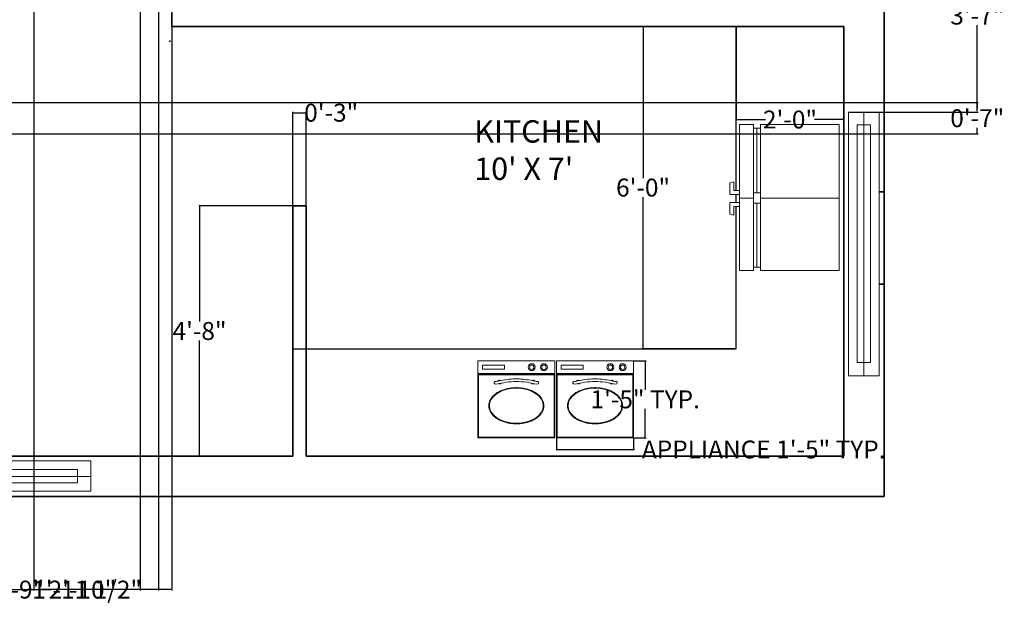
# Model space of a CAD drawing. Units: inches. Extents: x 311 to 754, y 60 to 497.
# Tile 6 of 11: x 530 to 750, y 60 to 194. Entities that reach past the tile are written whole.
import ezdxf

# ---------------------------------------------------------------- set-up
doc = ezdxf.new("R2010")
doc.units = ezdxf.units.IN
doc.header["$MEASUREMENT"] = 0
for name, color, linetype, lineweight in [('A-ANNO-DIMS', 2, 'Continuous', 18), ('A-AREA-IDEN', 1, 'Continuous', 18), ('A-EQPM', 8, 'Continuous', 18), ('A-FLOR-CASE', 30, 'Continuous', 25), ('A-WALL', 7, 'Continuous', 35), ('windows', 120, 'Continuous', 18)]:
    doc.layers.add(name, color=color, linetype=linetype, lineweight=lineweight)
doc.styles.get("Standard").update_dxf_attribs({"font": 'arial.ttf'})
doc.dimstyles.get("Standard").update_dxf_attribs({"dimtxt": 4, "dimasz": 0.18, "dimexe": 0.18, "dimexo": 0.0625, "dimgap": 0.09, "dimtad": 0, "dimtih": 1, "dimtoh": 1, "dimdec": 0, "dimrnd": 6, "dimzin": 0, "dimdsep": 46, "dimlunit": 3, "dimtxsty": 'Standard', "dimcen": 0.09, "dimadec": 0, "dimazin": 0, "dimtfac": 1, "dimtdec": 0, "dimtofl": 0, "dimtmove": 0, "dimatfit": 3, "dimfxl": 1, "dimtolj": 1, "dimtzin": 0, "dimarcsym": 0})

# ---------------------------------------------------------------- blocks, each defined once
blk = doc.blocks.new('A$C7E884C79')
for p, q in [((0, 0), (0, 600)), ((0, 600), (0, 0)), ((0, 600), (600, 600)), ((600, 600), (600, 0)), ((600, 0), (600, 600)), ((600, 600), (600, 450)), ((600, 600), (600, 500)), ((600, 500), (0, 500)), ((600, 495), (0, 495)), ((600, 500), (600, 0)), ((0, 0), (600, 0))]:
    blk.add_line(p, q)
for points in [[(36.4, 564.7), (208.9, 564.7), (208.9, 535.3), (36.4, 535.3)], [(5, 490), (595, 490), (595, 5), (5, 5)]]:
    blk.add_lwpolyline(points, close=True)
for centre, radius in [((419.3, 550), 27), ((419.3, 550), 17), ((513.9, 550), 27), ((513.9, 550), 17)]:
    blk.add_circle(centre, radius)
for centre, radius, start, end in [((137.2, 428), 10, 107.98291, 276.95811), ((168.5, 434.2), 15, 50.78881, 150.36701), ((168.5, 434.2), 15, 234.01645, 327.14121), ((431.5, 434.2), 15, 212.85879, 305.98355), ((431.5, 434.2), 15, 29.63299, 129.21119), ((462.8, 428), 10, 263.04189, 72.01709)]:
    blk.add_arc(centre, radius, start, end)
blk.add_ellipse((300, 250), major_axis=(-209.5, 0), ratio=0.648352)
for points, knots in [([(85.5, 250), (85.5, 244.8), (85.9, 239.6), (88, 226.9), (90.2, 219.4), (96.4, 204.8), (100.4, 197.7), (109.9, 184.1), (115.6, 177.5), (128.3, 165.1), (135.4, 159.2), (150.9, 148.3), (159.3, 143.3), (177.1, 134.2), (186.6, 130.1), (206.5, 123), (216.8, 119.9), (238.1, 114.9), (249, 113), (271.2, 110.2), (282.5, 109.4), (305, 109), (316.4, 109.4), (338.8, 111.3), (349.8, 112.8), (371.5, 117), (382.1, 119.6), (402.5, 126), (412.3, 129.7), (431, 138.1), (439.8, 142.8), (456.2, 153), (463.8, 158.6), (477.6, 170.5), (483.8, 176.8), (494.6, 190.1), (499.2, 197), (506.7, 211.3), (509.5, 218.7), (513.4, 233.6), (514.4, 241.3), (514.6, 256.5), (513.8, 264.1), (510.2, 279.1), (507.6, 286.6), (500.4, 300.9), (496, 307.9), (485.5, 321.3), (479.5, 327.7), (466, 339.7), (458.5, 345.3), (442.4, 355.8), (433.6, 360.5), (415.2, 369.1), (405.5, 373), (385.2, 379.5), (374.7, 382.3), (353.1, 386.7), (342, 388.3), (319.7, 390.5), (308.4, 390.9), (285.8, 390.7), (274.5, 390.1), (252.3, 387.5), (241.3, 385.7), (219.9, 380.9), (209.5, 378), (189.5, 371), (179.9, 367.1), (161.8, 358.1), (153.3, 353.2), (137.6, 342.5), (130.3, 336.7), (117.3, 324.4), (111.6, 317.9), (101.6, 304.3), (97.5, 297.3), (91, 282.8), (88.6, 275.3), (86, 261.9), (85.5, 255.9), (85.5, 250)], [0, 0, 0, 0, 0.108301, 0.108301, 0.267534, 0.267534, 0.426768, 0.426768, 0.586002, 0.586002, 0.745235, 0.745235, 0.904469, 0.904469, 1.063703, 1.063703, 1.222936, 1.222936, 1.38217, 1.38217, 1.541404, 1.541404, 1.700637, 1.700637, 1.859871, 1.859871, 2.019105, 2.019105, 2.178339, 2.178339, 2.337572, 2.337572, 2.496806, 2.496806, 2.65604, 2.65604, 2.815273, 2.815273, 2.974507, 2.974507, 3.133741, 3.133741, 3.292974, 3.292974, 3.452208, 3.452208, 3.611442, 3.611442, 3.770676, 3.770676, 3.929909, 3.929909, 4.089143, 4.089143, 4.248377, 4.248377, 4.40761, 4.40761, 4.566844, 4.566844, 4.726078, 4.726078, 4.885311, 4.885311, 5.044545, 5.044545, 5.203779, 5.203779, 5.363012, 5.363012, 5.522246, 5.522246, 5.68148, 5.68148, 5.840714, 5.840714, 5.999947, 5.999947, 6.159181, 6.159181, 6.283185, 6.283185, 6.283185, 6.283185]), ([(134.1, 437.5), (144.6, 439.5), (155.1, 441.6), (186, 447.3), (206.5, 450.9), (247.9, 456.4), (268.7, 458.3), (293.5, 458.9), (297.3, 458.9), (304.8, 458.9), (308.5, 458.8), (319.7, 458.5), (327.1, 458.1), (349.4, 456.5), (364.1, 454.9), (399.8, 449.9), (420.6, 446.2), (449.5, 440.7), (457.7, 439.1), (465.9, 437.5)], [0, 0, 0, 0, 31.638865, 31.638865, 92.600143, 92.600143, 153.561421, 153.561421, 164.367647, 164.367647, 175.173874, 175.173874, 196.786327, 196.786327, 240.011233, 240.011233, 302.099201, 302.099201, 326.773065, 326.773065, 326.773065, 326.773065])]:
    blk.add_open_spline(points, degree=3, knots=knots)
blk.add_open_spline([(138, 417.8), (192, 428.4), (300, 449.4), (408, 428.4), (462, 417.8)], degree=3)
blk = doc.blocks.new('WIN-FRAME-59IN')
for points in [[(0, 0), (0, 6.8), (58.92, 6.8), (58.92, 0)], [(2.85, 4.84), (55.97, 4.84), (55.97, 1.89), (2.85, 1.89)]]:
    blk.add_lwpolyline(points, close=True)
blk = doc.blocks.new('*D112')
at = {"layer": 'A-ANNO-DIMS', "color": 0, "lineweight": -2, "transparency": 16777216}
for p, q in [((649.67, 100.26), (649.67, 97.56)), ((666.89, 100.26), (666.89, 97.56)), ((649.85, 97.74), (666.71, 97.74)), ((666.89, 97.74), (667.07, 97.74))]:
    blk.add_line(p, q, dxfattribs=at)
at = {"layer": 'A-ANNO-DIMS', "color": 0, "transparency": 16777216}
for points in [[(649.85, 97.77), (649.85, 97.71), (649.67, 97.74)], [(666.71, 97.77), (666.71, 97.71), (666.89, 97.74)]]:
    blk.add_solid(points, dxfattribs=at)
at = {"layer": 'Defpoints', "color": 0, "transparency": 16777216}
for p in [(649.67, 100.33), (666.89, 100.33), (666.89, 97.74)]:
    blk.add_point(p, dxfattribs=at)
at = {"layer": 'A-ANNO-DIMS', "color": 0, "transparency": 16777216, "insert": (695.93, 97.74), "char_height": 4, "attachment_point": 5}
blk.add_mtext('\\A1;APPLIANCE 1\'-5" TYP.', dxfattribs=at)
blk = doc.blocks.new('*D113')
at = {"layer": 'A-ANNO-DIMS', "color": 0, "lineweight": -2, "transparency": 16777216}
for p, q in [((666.95, 117.55), (669.66, 117.55)), ((669.48, 117.37), (669.48, 111.07)), ((669.48, 100.51), (669.48, 106.81)), ((666.95, 100.33), (669.66, 100.33))]:
    blk.add_line(p, q, dxfattribs=at)
at = {"layer": 'A-ANNO-DIMS', "color": 0, "transparency": 16777216}
for points in [[(669.45, 117.37), (669.51, 117.37), (669.48, 117.55)], [(669.45, 100.51), (669.51, 100.51), (669.48, 100.33)]]:
    blk.add_solid(points, dxfattribs=at)
at = {"layer": 'Defpoints', "color": 0, "transparency": 16777216}
for p in [(666.89, 117.55), (669.48, 117.55), (666.89, 100.33)]:
    blk.add_point(p, dxfattribs=at)
at = {"layer": 'A-ANNO-DIMS', "color": 0, "transparency": 16777216, "insert": (669.48, 108.94), "char_height": 4, "attachment_point": 5}
blk.add_mtext('\\A1;1\'-5" TYP.', dxfattribs=at)
blk = doc.blocks.new('*D123')
at = {"layer": 'A-ANNO-DIMS', "color": 0, "lineweight": -2, "transparency": 16777216}
for p, q in [((715.13, 216.2), (743.78, 216.2)), ((743.6, 216.02), (743.6, 196.79)), ((743.6, 173.28), (743.6, 192.52)), ((714.96, 173.1), (743.78, 173.1))]:
    blk.add_line(p, q, dxfattribs=at)
at = {"layer": 'A-ANNO-DIMS', "color": 0, "transparency": 16777216}
for points in [[(743.57, 216.02), (743.63, 216.02), (743.6, 216.2)], [(743.57, 173.28), (743.63, 173.28), (743.6, 173.1)]]:
    blk.add_solid(points, dxfattribs=at)
at = {"layer": 'Defpoints', "color": 0, "transparency": 16777216}
for p in [(715.07, 216.2), (714.89, 173.1), (743.6, 173.1)]:
    blk.add_point(p, dxfattribs=at)
at = {"layer": 'A-ANNO-DIMS', "color": 0, "transparency": 16777216, "insert": (743.6, 194.65), "char_height": 4, "attachment_point": 5}
blk.add_mtext('\\A1;3\'-7"', dxfattribs=at)
blk = doc.blocks.new('*D132')
at = {"layer": 'A-ANNO-DIMS', "color": 0, "lineweight": -2, "transparency": 16777216}
for p, q in [((526.91, 339.18), (526.91, 66.26)), ((560.82, 339.18), (560.82, 66.26)), ((527.09, 66.44), (536.87, 66.44)), ((560.64, 66.44), (550.86, 66.44))]:
    blk.add_line(p, q, dxfattribs=at)
at = {"layer": 'A-ANNO-DIMS', "color": 0, "transparency": 16777216}
for points in [[(527.09, 66.47), (527.09, 66.41), (526.91, 66.44)], [(560.64, 66.47), (560.64, 66.41), (560.82, 66.44)]]:
    blk.add_solid(points, dxfattribs=at)
at = {"layer": 'Defpoints', "color": 0, "transparency": 16777216}
for p in [(526.91, 339.24), (560.82, 339.24), (526.91, 66.44)]:
    blk.add_point(p, dxfattribs=at)
at = {"layer": 'A-ANNO-DIMS', "color": 0, "transparency": 16777216, "insert": (543.87, 66.44), "char_height": 4, "attachment_point": 5}
blk.add_mtext('\\A1;2\'-10"', dxfattribs=at)
blk = doc.blocks.new('*D133')
at = {"layer": 'A-ANNO-DIMS', "color": 0, "lineweight": -2, "transparency": 16777216}
for p, q in [((590.8, 152.22), (590.8, 173.14)), ((590.98, 172.96), (593.62, 172.96)), ((593.8, 152.22), (593.8, 173.14)), ((593.8, 172.96), (593.98, 172.96))]:
    blk.add_line(p, q, dxfattribs=at)
at = {"layer": 'A-ANNO-DIMS', "color": 0, "transparency": 16777216}
for points in [[(590.98, 172.99), (590.98, 172.93), (590.8, 172.96)], [(593.62, 172.99), (593.62, 172.93), (593.8, 172.96)]]:
    blk.add_solid(points, dxfattribs=at)
at = {"layer": 'Defpoints', "color": 0, "transparency": 16777216}
for p in [(593.8, 172.96), (590.8, 152.16), (593.8, 152.16)]:
    blk.add_point(p, dxfattribs=at)
at = {"layer": 'A-ANNO-DIMS', "color": 0, "transparency": 16777216, "insert": (599.39, 172.96), "char_height": 4, "attachment_point": 5}
blk.add_mtext('\\A1;0\'-3"', dxfattribs=at)
blk = doc.blocks.new('*D134')
at = {"layer": 'A-ANNO-DIMS', "color": 0, "lineweight": -2, "transparency": 16777216}
for p, q in [((494.8, 342.18), (494.8, 66.26)), ((563.8, 342.18), (563.8, 66.26)), ((494.98, 66.44), (523.9, 66.44)), ((563.62, 66.44), (534.71, 66.44))]:
    blk.add_line(p, q, dxfattribs=at)
at = {"layer": 'A-ANNO-DIMS', "color": 0, "transparency": 16777216}
for points in [[(494.98, 66.47), (494.98, 66.41), (494.8, 66.44)], [(563.62, 66.47), (563.62, 66.41), (563.8, 66.44)]]:
    blk.add_solid(points, dxfattribs=at)
at = {"layer": 'Defpoints', "color": 0, "transparency": 16777216}
for p in [(494.8, 342.24), (563.8, 342.24), (563.8, 66.44)]:
    blk.add_point(p, dxfattribs=at)
at = {"layer": 'A-ANNO-DIMS', "color": 0, "transparency": 16777216, "insert": (529.3, 66.44), "char_height": 4, "attachment_point": 5}
blk.add_mtext('\\A1;5\'-9"', dxfattribs=at)
blk = doc.blocks.new('*D135')
at = {"layer": 'A-ANNO-DIMS', "color": 0, "lineweight": -2, "transparency": 16777216}
for p, q in [((590.74, 152.16), (569.82, 152.16)), ((570, 151.98), (570, 126.33)), ((570, 96.42), (570, 122.07)), ((590.74, 96.24), (569.82, 96.24))]:
    blk.add_line(p, q, dxfattribs=at)
at = {"layer": 'A-ANNO-DIMS', "color": 0, "transparency": 16777216}
for points in [[(569.97, 151.98), (570.03, 151.98), (570, 152.16)], [(569.97, 96.42), (570.03, 96.42), (570, 96.24)]]:
    blk.add_solid(points, dxfattribs=at)
at = {"layer": 'Defpoints', "color": 0, "transparency": 16777216}
for p in [(570, 152.16), (590.8, 152.16), (590.8, 96.24)]:
    blk.add_point(p, dxfattribs=at)
at = {"layer": 'A-ANNO-DIMS', "color": 0, "transparency": 16777216, "insert": (570, 124.2), "char_height": 4, "attachment_point": 5}
blk.add_mtext('\\A1;4\'-8"', dxfattribs=at)
blk = doc.blocks.new('*D141')
at = {"layer": 'A-ANNO-DIMS', "color": 0, "lineweight": -2, "transparency": 16777216}
for p, q in [((449.87, 175.24), (743.78, 175.24)), ((743.6, 175.06), (743.6, 173.87)), ((743.6, 168.42), (743.6, 169.61)), ((449.87, 168.24), (743.78, 168.24))]:
    blk.add_line(p, q, dxfattribs=at)
at = {"layer": 'A-ANNO-DIMS', "color": 0, "transparency": 16777216}
for points in [[(743.57, 175.06), (743.63, 175.06), (743.6, 175.24)], [(743.57, 168.42), (743.63, 168.42), (743.6, 168.24)]]:
    blk.add_solid(points, dxfattribs=at)
at = {"layer": 'Defpoints', "color": 0, "transparency": 16777216}
for p in [(449.8, 175.24), (743.6, 175.24), (449.8, 168.24)]:
    blk.add_point(p, dxfattribs=at)
at = {"layer": 'A-ANNO-DIMS', "color": 0, "transparency": 16777216, "insert": (743.6, 171.74), "char_height": 4, "attachment_point": 5}
blk.add_mtext('\\A1;0\'-7"', dxfattribs=at)
blk = doc.blocks.new('*D142')
at = {"layer": 'A-ANNO-DIMS', "color": 0, "lineweight": -2, "transparency": 16777216}
for p, q in [((689.8, 192.18), (689.8, 171.26)), ((713.8, 192.18), (713.8, 171.26)), ((689.98, 171.44), (696.36, 171.44)), ((713.62, 171.44), (707.25, 171.44))]:
    blk.add_line(p, q, dxfattribs=at)
at = {"layer": 'A-ANNO-DIMS', "color": 0, "transparency": 16777216}
for points in [[(689.98, 171.47), (689.98, 171.41), (689.8, 171.44)], [(713.62, 171.47), (713.62, 171.41), (713.8, 171.44)]]:
    blk.add_solid(points, dxfattribs=at)
at = {"layer": 'Defpoints', "color": 0, "transparency": 16777216}
for p in [(689.8, 192.24), (713.8, 192.24), (689.8, 171.44)]:
    blk.add_point(p, dxfattribs=at)
at = {"layer": 'A-ANNO-DIMS', "color": 0, "transparency": 16777216, "insert": (701.8, 171.44), "char_height": 4, "attachment_point": 5}
blk.add_mtext('\\A1;2\'-0"', dxfattribs=at)
blk = doc.blocks.new('*D143')
at = {"layer": 'A-ANNO-DIMS', "color": 0, "lineweight": -2, "transparency": 16777216}
for p, q in [((689.74, 192.24), (668.82, 192.24)), ((669, 192.06), (669, 158.37)), ((669, 120.42), (669, 154.11)), ((689.74, 120.24), (668.82, 120.24))]:
    blk.add_line(p, q, dxfattribs=at)
at = {"layer": 'A-ANNO-DIMS', "color": 0, "transparency": 16777216}
for points in [[(668.97, 192.06), (669.03, 192.06), (669, 192.24)], [(668.97, 120.42), (669.03, 120.42), (669, 120.24)]]:
    blk.add_solid(points, dxfattribs=at)
at = {"layer": 'Defpoints', "color": 0, "transparency": 16777216}
for p in [(669, 192.24), (689.8, 192.24), (689.8, 120.24)]:
    blk.add_point(p, dxfattribs=at)
at = {"layer": 'A-ANNO-DIMS', "color": 0, "transparency": 16777216, "insert": (669, 156.24), "char_height": 4, "attachment_point": 5}
blk.add_mtext('\\A1;6\'-0"', dxfattribs=at)
blk = doc.blocks.new('*D146')
at = {"layer": 'A-ANNO-DIMS', "color": 0, "lineweight": -2, "transparency": 16777216}
for p, q in [((533.04, 385.85), (533.04, 66.26)), ((556.78, 385.85), (556.78, 66.26)), ((533.22, 66.44), (533.47, 66.44)), ((556.6, 66.44), (556.34, 66.44))]:
    blk.add_line(p, q, dxfattribs=at)
at = {"layer": 'A-ANNO-DIMS', "color": 0, "transparency": 16777216}
for points in [[(533.22, 66.47), (533.22, 66.41), (533.04, 66.44)], [(556.6, 66.47), (556.6, 66.41), (556.78, 66.44)]]:
    blk.add_solid(points, dxfattribs=at)
at = {"layer": 'Defpoints', "color": 0, "transparency": 16777216}
for p in [(533.04, 385.92), (556.78, 385.92), (556.78, 66.44)]:
    blk.add_point(p, dxfattribs=at)
at = {"layer": 'A-ANNO-DIMS', "color": 0, "transparency": 16777216, "insert": (544.91, 66.44), "char_height": 4, "attachment_point": 5}
blk.add_mtext('\\A1;1\'-11 1/2"', dxfattribs=at)
blk = doc.blocks.new('*D156')
at = {"layer": 'A-ANNO-DIMS', "color": 0, "lineweight": -2, "transparency": 16777216}
for p, q in [((604.46, 239.76), (589.17, 220.85)), ((604.64, 239.76), (604.46, 239.76)), ((563.4, 188.88), (563.4, 189.06)), ((563.31, 188.97), (563.49, 188.97))]:
    blk.add_line(p, q, dxfattribs=at)
at = {"layer": 'A-ANNO-DIMS', "color": 0, "transparency": 16777216}
blk.add_solid([(589.15, 220.87), (589.2, 220.83), (589.06, 220.71)], dxfattribs=at)
at = {"layer": 'Defpoints', "color": 0, "transparency": 16777216}
for p in [(589.06, 220.71), (563.4, 188.97)]:
    blk.add_point(p, dxfattribs=at)
at = {"layer": 'A-ANNO-DIMS', "color": 0, "transparency": 16777216, "insert": (611.96, 239.76), "char_height": 4, "attachment_point": 5}
blk.add_mtext('\\A1;R3\'-5"', dxfattribs=at)

msp = doc.modelspace()

# ---------------------------------------------------------------- linework, layer by layer
at = {"layer": 'A-EQPM'}
for p, q in [((693.63, 169.51), (695.2, 169.51)), ((694.42, 155.08), (694.42, 169.51)), ((693.63, 153.89), (690.49, 153.89)), ((693.63, 155.08), (695.2, 155.08)), ((712.74, 153.89), (695.2, 153.89)), ((693.63, 152.76), (695.2, 152.76)), ((694.42, 138.47), (694.42, 152.76)), ((695.2, 138.47), (693.63, 138.47))]:
    msp.add_line(p, q, dxfattribs=at)
for points in [[(693.63, 170.3), (693.63, 137.69), (690.49, 137.69), (690.49, 170.3)], [(712.74, 170.3), (712.74, 137.69), (695.2, 137.69), (695.2, 170.3)], [(688.37, 154.72), (690.49, 154.72), (690.49, 155.6), (689.25, 155.6), (689.25, 157.54), (688.37, 157.31)]]:
    msp.add_lwpolyline(points, close=True, dxfattribs=at)
msp.add_lwpolyline([(690.49, 152.02), (689.25, 152.02), (689.25, 150.08), (688.37, 150.31), (688.37, 152.9), (690.49, 152.9)], dxfattribs=at)
at = {"layer": 'A-FLOR-CASE'}
for p, q in [((689.8, 155.6), (689.8, 192.24)), ((689.8, 152.9), (689.8, 154.72)), ((689.8, 120.24), (689.8, 152.02)), ((590.8, 120.24), (689.8, 120.24))]:
    msp.add_line(p, q, dxfattribs=at)
at = {"layer": 'A-WALL'}
for p, q in [((722.8, 87.24), (722.8, 447.24)), ((563.8, 192.24), (563.8, 195.24)), ((713.8, 192.24), (563.8, 192.24)), ((713.8, 96.24), (713.8, 192.24)), ((722.8, 155.29), (721.7, 155.29)), ((590.8, 96.24), (590.8, 152.16)), ((590.8, 96.24), (590.8, 152.16)), ((590.8, 152.16), (593.8, 152.16)), ((593.8, 96.24), (593.8, 152.16)), ((722.8, 134.69), (721.7, 134.69)), ((443.8, 96.24), (590.8, 96.24)), ((593.8, 96.24), (713.8, 96.24)), ((443.8, 87.24), (722.8, 87.24))]:
    msp.add_line(p, q, dxfattribs=at)
at = {"layer": 'windows'}
for p, q in [((714.89, 173.1), (718.26, 173.1)), ((718.26, 173.1), (718.26, 114.18)), ((718.26, 114.18), (717.32, 114.18)), ((545.72, 91.7), (486.8, 91.7)), ((545.72, 88.42), (545.72, 91.7))]:
    msp.add_line(p, q, dxfattribs=at)

# ---------------------------------------------------------------- block references
at = {"layer": 'A-EQPM', "xscale": 0.0287068133738272, "yscale": 0.0287068133738272, "zscale": 0.0287068133738272}
for p in [(632.11, 100.33), (649.67, 100.33)]:
    msp.add_blockref('A$C7E884C79', p, dxfattribs=at)
at = {"layer": 'windows', "rotation": 269.9999999999999}
msp.add_blockref('WIN-FRAME-59IN', (714.89, 173.1), dxfattribs=at)
at = {"layer": 'windows'}
msp.add_blockref('WIN-FRAME-59IN', (486.8, 88.42), dxfattribs=at)

# ---------------------------------------------------------------- texts
at = {"layer": 'A-AREA-IDEN', "ltscale": 50, "insert": (631.31, 171.28), "char_height": 5, "attachment_point": 1}
msp.add_mtext_dynamic_manual_height_columns("KITCHEN\\P10' X 7'\\P ", width=51.3734, gutter_width=1, heights=[0], dxfattribs=at)

# ---------------------------------------------------------------- dimensions: what is measured, and where the dimension line sits
at = {"layer": 'A-ANNO-DIMS'}
for base, p1, p2, picture, middle in [((556.78, 66.44), (533.04, 385.92), (556.78, 385.92), '*D146', (544.91, 66.44)), ((563.8, 66.44), (494.8, 342.24), (563.8, 342.24), '*D134', (529.3, 66.44)), ((526.91, 66.44), (560.82, 339.24), (526.91, 339.24), '*D132', (543.87, 66.44)), ((593.8, 172.96), (590.8, 152.16), (593.8, 152.16), '*D133', (599.39, 172.96))]:
    dim = msp.add_linear_dim(base=base, p1=p1, p2=p2, dimstyle='Standard', override={"dimdec": 1, "dimlfac": 1, "dimrnd": 0, "dimzin": 1, "dimdsep": 46, "dimlunit": 4, "dimfrac": 2}, dxfattribs=at)
    dim.commit()
    dim.dimension.update_dxf_attribs({"geometry": picture, "text_midpoint": middle})
dim = msp.add_radius_dim(center=(563.4, 188.97), mpoint=(589.06, 220.71), dimstyle='Standard', override={"dimdec": 1, "dimlfac": 1, "dimrnd": 0, "dimzin": 1, "dimdsep": 46, "dimlunit": 4, "dimfrac": 2}, dxfattribs=at)
dim.commit()
dim.dimension.update_dxf_attribs({"geometry": '*D156', "text_midpoint": (611.96, 239.76), "dimtype": 164})
for base, p1, p2, angle, picture, middle in [((743.6, 173.1), (715.07, 216.2), (714.89, 173.1), 90, '*D123', (743.6, 194.65)), ((669, 192.24), (689.8, 120.24), (689.8, 192.24), 90, '*D143', (669, 156.24)), ((689.8, 171.44), (713.8, 192.24), (689.8, 192.24), 180, '*D142', (701.8, 171.44)), ((743.6, 175.24), (449.8, 168.24), (449.8, 175.24), 90, '*D141', (743.6, 171.74)), ((570, 152.16), (590.8, 96.24), (590.8, 152.16), 90, '*D135', (570, 124.2))]:
    dim = msp.add_linear_dim(base=base, p1=p1, p2=p2, angle=angle, dimstyle='Standard', override={"dimdec": 1, "dimlfac": 1, "dimrnd": 0, "dimzin": 1, "dimdsep": 46, "dimlunit": 4, "dimfrac": 2}, dxfattribs=at)
    dim.commit()
    dim.dimension.update_dxf_attribs({"geometry": picture, "text_midpoint": middle})
dim = msp.add_linear_dim(base=(669.48, 117.55), p1=(666.89, 100.33), p2=(666.89, 117.55), angle=90, text='<> TYP.', dimstyle='Standard', override={"dimdec": 1, "dimlfac": 1, "dimrnd": 0, "dimzin": 1, "dimdsep": 46, "dimlunit": 4, "dimfrac": 2}, dxfattribs=at)
dim.commit()
dim.dimension.update_dxf_attribs({"geometry": '*D113', "text_midpoint": (669.48, 108.94)})
dim = msp.add_linear_dim(base=(666.89, 97.74), p1=(649.67, 100.33), p2=(666.89, 100.33), text='APPLIANCE <> TYP.', dimstyle='Standard', override={"dimdec": 1, "dimlfac": 1, "dimrnd": 0, "dimzin": 1, "dimdsep": 46, "dimlunit": 4, "dimfrac": 2}, dxfattribs=at)
dim.commit()
dim.dimension.update_dxf_attribs({"geometry": '*D112', "text_midpoint": (695.93, 97.74)})

doc.saveas('drawing.dxf')
